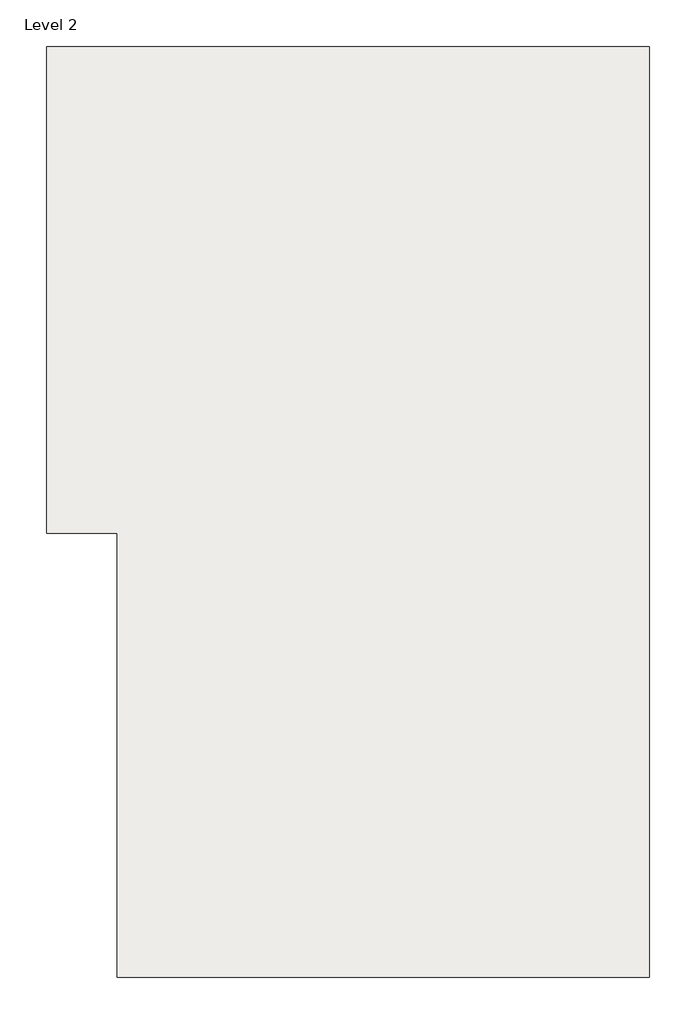
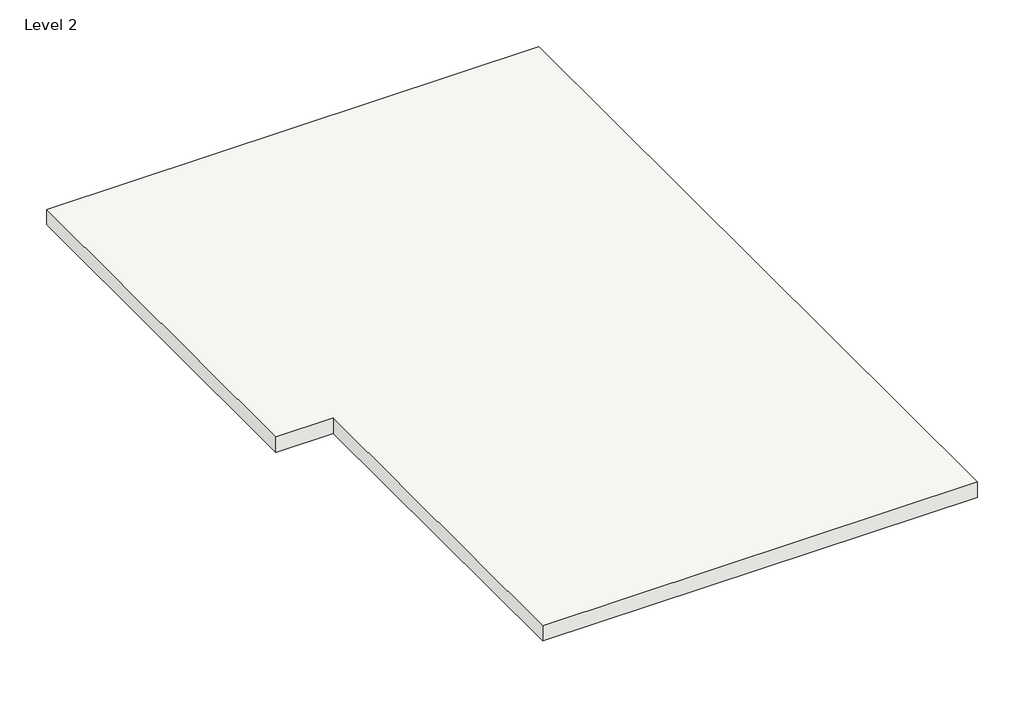
# One storey: 1 roof.
"""IFC4 building model written with IfcOpenShell, lengths in millimetres."""

from ifc_helpers import new_model, si_unit, frame, origin, place, context, project, spatial, polyline, outline, extrude, element, save

model = new_model("IFC4")

# Units and contexts
model_context = context("Model", 3, world=origin())
ifc_project = project(units=[si_unit("LENGTHUNIT", "METRE", prefix="MILLI")], contexts=[model_context])

# Site, building, storey
site = spatial("IfcSite", under=ifc_project)
building = spatial("IfcBuilding", under=site)
storey = spatial("IfcBuildingStorey", under=building, Name="Level 2", Elevation=3048.0)

# Roof
placement = place(None, origin())
element("IfcRoof", 1, ObjectType="Generic - 12\"", at=placement, inside=storey, context=model_context, shape_type="SweptSolid", body=[
    extrude(outline(polyline([(-11912.8247577, 14369.953629), (-2565.6247577, 14369.953629), (-2565.6247577, -57.246371), (-10820.6247577, -57.246371), (-10820.6247577, 6826.153629), (-11912.8247577, 6826.153629), (-11912.8247577, 14369.953629)])), frame((0.0, 0.0, 3048.0), z_axis=(0.0, 0.0, 1.0), x_axis=(1.0, 0.0, 0.0)), (0.0, 0.0, 1.0), 304.8),
])

save(model, "model.ifc")

# Revit data of these elements
# Type "Generic - 12\""
#   Assembly Code = "B1020"
#   Layers, outside or top first: 1' - 0" "Brick, Soldier Course" (function 1)
# Element 1 (IfcRoof, "Generic - 12\"")
#   built-in parameter 1001705 = 11 (stored number, unit not read)
#   built-in parameter 1001710 = 33615
#   Phase Created = New Construction
#   Materials on its faces: "Brick, Soldier Course"
# Materials
#   "Brick, Soldier Course": class "Masonry", colour RGB 170 98 104, transparency 0, Description = "Common brick soldier coursed", Cost = 0
